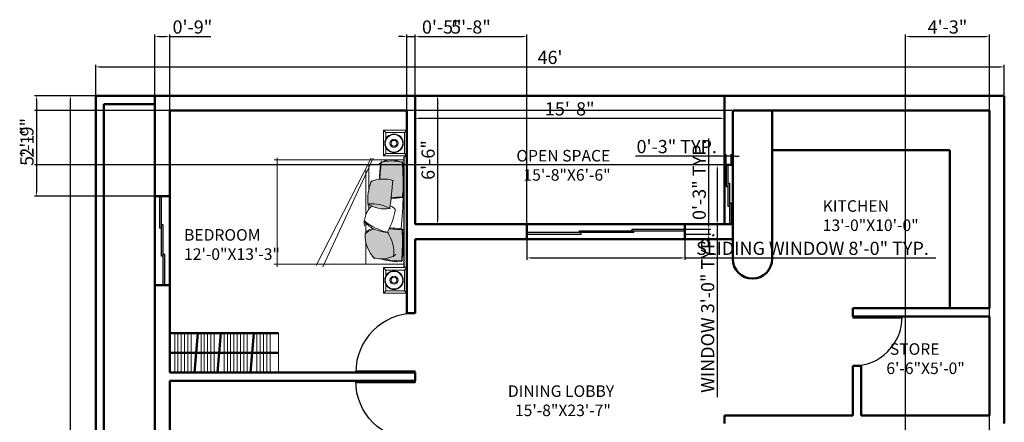
# Model space of a CAD drawing. Units: inches. Extents: x 1913 to 5309, y 1003 to 1733.
# Tile 8 of 23: x 1913 to 2511, y 1489 to 1733. Entities that reach past the tile are written whole.
import ezdxf

# ---------------------------------------------------------------- set-up
doc = ezdxf.new("R2010")
doc.units = ezdxf.units.IN
for name, color, linetype, lineweight in [('0.10', 252, 'Continuous', 9), ('0.15', 34, 'Continuous', 15), ('A-ANNO-DIMS', 2, 'Continuous', 18), ('A-AREA-IDEN', 3, 'Continuous', 18), ('A-DOOR', 4, 'Continuous', 25), ('A-FURN', 8, 'Continuous', 18), ('A-FURN-PATT', 8, 'Continuous', 13), ('A-GLAZ', 5, 'Continuous', 25), ('A-WALL', 7, 'Continuous', 50)]:
    doc.layers.add(name, color=color, linetype=linetype, lineweight=lineweight)
doc.styles.get("Standard").update_dxf_attribs({"font": 'arial.ttf'})
doc.dimstyles.new('ISO-25', dxfattribs={"dimtxt": 8, "dimasz": 2.5, "dimexe": 1.25, "dimexo": 0.625, "dimtad": 1, "dimdec": 1, "dimlunit": 3, "dimtxsty": 'Standard', "dimcen": 2.5, "dimclrd": 256, "dimclrt": 1, "dimadec": 0, "dimazin": 0, "dimtfac": 1, "dimtdec": 1, "dimtmove": 0, "dimatfit": 3, "dimfxl": 1, "dimarcsym": 0})

# ---------------------------------------------------------------- blocks, each defined once
blk = doc.blocks.new("D1 3'")
for p, q in [((0, 36), (0, 0)), ((1, 36), (1, 0)), ((0, 0), (1, 0))]:
    blk.add_line(p, q)
blk.add_arc((0, 0), 36, 0, 90)
blk = doc.blocks.new('camita')
at = {"layer": '0.10'}
for p, q in [((-0.85, -0.045), (0.85, -0.045)), ((-0.805, -0.045), (-0.805, -2.048)), ((0.805, -0.045), (0.805, -2.048)), ((-0.827, -0.521), (0.846, -1.293)), ((-0.827, -0.548), (0.824, -1.399)), ((-0.716, -0.585), (-0.355, -0.585)), ((-0.114, -0.585), (-0.049, -0.585)), ((-0.638, -0.63), (0.043, -0.63)), ((0.175, -0.63), (0.318, -0.63)), ((0.474, -0.63), (0.805, -0.63)), ((-0.835, -2), (0.846, -2))]:
    blk.add_line(p, q, dxfattribs=at)
blk.add_lwpolyline([(-0.85, -0.041), (0.85, -0.041), (0.85, 0), (-0.85, 0)], close=True, dxfattribs=at)
for centre, radius, start, end in [((-0.457, -0.236), 0.344, 147.51, 213.8336), ((-0.2, -0.227), 0.586, 163.9263, 197.1409), ((-0.364, -5.846), 5.791, 83.8073, 94.1211), ((-0.51, -1.723), 1.678, 80.1255, 98.6619), ((2.353, -0.053), 2.58, 180.1063, 184.3854), ((-1.544, -0.245), 1.333, 359.9394, 7.5533), ((1.581, -0.289), 1.335, 170.3802, 178.9914), ((-1.44, -0.061), 1.712, 352.9291, 0.3959), ((0.452, -3.067), 3, 83.9026, 93.6759), ((0.486, -1.629), 1.578, 80.1602, 98.06), ((0.029, -0.138), 0.726, 342.5841, 6.0048), ((0.133, -0.17), 0.631, 339.923, 8.7433), ((-0.054, -0.363), 0.454, 159.3026, 206.5026), ((-1.33, -9.675), 9.499, 82.2708, 84.9399), ((0.458, -0.545), 0.584, 151.0456, 184.1497), ((-0.534, -0.339), 0.487, 327.2644, 9.0473), ((-0.007, -0.258), 0.0828, 100.018, 179.736), ((-0.293, -1.438), 1.29, 61.9749, 77.8435), ((-0.199, -0.274), 0.516, 310.7395, 359.0576), ((-0.567, -0.087), 0.906, 321.6953, 346.4626), ((0.627, -0.752), 0.551, 82.9691, 124.6739), ((0.32, -0.394), 0.404, 341.4524, 33.4512), ((-1.867, -14.986), 14.632, 84.6597, 85.7516), ((-0.46, 1.486), 1.909, 260.953, 268.6517), ((-0.2, 0.064), 0.667, 244.7809, 279.0606), ((0.179, -0.272), 0.383, 224.5284, 275.2229), ((0.438, -0.483), 0.19, 193.6849, 236.7035), ((0.571, -0.432), 0.315, 192.9388, 221.9636), ((0.361, -0.133), 0.51, 267.2589, 315.2997)]:
    blk.add_arc(centre, radius, start, end, dxfattribs=at)
blk = doc.blocks.new('VELADOR')
at = {"layer": '0.15'}
for p, q in [((-0.248, 0), (-0.203, -0.045)), ((0.248, 0), (0.202, -0.045)), ((-0.203, -0.405), (-0.248, -0.45)), ((0.248, -0.45), (0.202, -0.405))]:
    blk.add_line(p, q, dxfattribs=at)
blk.add_lwpolyline([(-0.248, 0), (-0.248, -0.45), (0.248, -0.45), (0.248, 0)], close=True, dxfattribs=at)
blk.add_lwpolyline([(0.092, -0.405), (0.202, -0.405), (0.202, -0.045), (-0.203, -0.045), (-0.203, -0.405), (-0.082, -0.405)], dxfattribs=at)
for radius in [0.18, 0.169, 0.0788, 0.0563]:
    blk.add_circle((0.005, -0.247), radius, dxfattribs=at)
blk = doc.blocks.new('*D20')
at = {"layer": 'A-ANNO-DIMS', "color": 0, "lineweight": -2, "transparency": 16777216}
for p, q in [((1958.75, 1686.96), (1942.76, 1686.96)), ((1944.01, 1101.46), (1944.01, 1684.46)), ((1958.75, 1098.96), (1942.76, 1098.96))]:
    blk.add_line(p, q, dxfattribs=at)
at = {"layer": 'A-ANNO-DIMS', "color": 0, "transparency": 16777216}
for points in [[(1943.6, 1684.46), (1944.43, 1684.46), (1944.01, 1686.96)], [(1943.6, 1101.46), (1944.43, 1101.46), (1944.01, 1098.96)]]:
    blk.add_solid(points, dxfattribs=at)
at = {"layer": 'Defpoints', "color": 0, "transparency": 16777216}
for p in [(1944.01, 1686.96), (1959.37, 1686.96), (1959.37, 1098.96)]:
    blk.add_point(p, dxfattribs=at)
at = {"layer": 'A-ANNO-DIMS', "color": 0, "transparency": 16777216, "insert": (1939.3, 1392.96), "char_height": 8, "attachment_point": 5, "rotation": 90}
blk.add_mtext("49'", dxfattribs=at)
blk = doc.blocks.new('*D22')
at = {"layer": 'A-ANNO-DIMS', "color": 0, "lineweight": -2, "transparency": 16777216}
for p, q in [((1959.37, 1687.59), (1959.37, 1705.75)), ((2511.37, 1687.59), (2511.37, 1705.75)), ((1961.87, 1704.5), (2508.87, 1704.5))]:
    blk.add_line(p, q, dxfattribs=at)
at = {"layer": 'A-ANNO-DIMS', "color": 0, "transparency": 16777216}
for points in [[(1961.87, 1704.92), (1961.87, 1704.08), (1959.37, 1704.5)], [(2508.87, 1704.92), (2508.87, 1704.08), (2511.37, 1704.5)]]:
    blk.add_solid(points, dxfattribs=at)
at = {"layer": 'Defpoints', "color": 0, "transparency": 16777216}
for p in [(2511.37, 1704.5), (1959.37, 1686.96), (2511.37, 1686.96)]:
    blk.add_point(p, dxfattribs=at)
at = {"layer": 'A-ANNO-DIMS', "color": 0, "transparency": 16777216, "insert": (2235.37, 1709.21), "char_height": 8, "attachment_point": 5}
blk.add_mtext("46'", dxfattribs=at)
blk = doc.blocks.new('*D23')
at = {"layer": 'A-ANNO-DIMS', "color": 0, "lineweight": -2, "transparency": 16777216}
for p, q in [((2153.37, 1679.78), (2153.37, 1672.02)), ((2341.37, 1679.78), (2341.37, 1672.02)), ((2155.87, 1673.27), (2338.87, 1673.27))]:
    blk.add_line(p, q, dxfattribs=at)
at = {"layer": 'A-ANNO-DIMS', "color": 0, "transparency": 16777216}
for points in [[(2155.87, 1673.68), (2155.87, 1672.85), (2153.37, 1673.27)], [(2338.87, 1673.68), (2338.87, 1672.85), (2341.37, 1673.27)]]:
    blk.add_solid(points, dxfattribs=at)
at = {"layer": 'Defpoints', "color": 0, "transparency": 16777216}
for p in [(2153.37, 1680.41), (2341.37, 1680.41), (2341.37, 1673.27)]:
    blk.add_point(p, dxfattribs=at)
at = {"layer": 'A-ANNO-DIMS', "color": 0, "transparency": 16777216, "insert": (2247.37, 1677.98), "char_height": 8, "attachment_point": 5}
blk.add_mtext('15\'-8"', dxfattribs=at)
blk = doc.blocks.new('*D24')
at = {"layer": 'A-ANNO-DIMS', "color": 0, "lineweight": -2, "transparency": 16777216}
for p, q in [((2167.19, 1686.96), (2165.81, 1686.96)), ((2167.06, 1684.46), (2167.06, 1611.46)), ((2167.19, 1608.96), (2165.81, 1608.96))]:
    blk.add_line(p, q, dxfattribs=at)
at = {"layer": 'A-ANNO-DIMS', "color": 0, "transparency": 16777216}
for points in [[(2166.65, 1684.46), (2167.48, 1684.46), (2167.06, 1686.96)], [(2166.65, 1611.46), (2167.48, 1611.46), (2167.06, 1608.96)]]:
    blk.add_solid(points, dxfattribs=at)
at = {"layer": 'Defpoints', "color": 0, "transparency": 16777216}
for p in [(2167.81, 1686.96), (2167.06, 1608.96), (2167.81, 1608.96)]:
    blk.add_point(p, dxfattribs=at)
at = {"layer": 'A-ANNO-DIMS', "color": 0, "transparency": 16777216, "insert": (2162.35, 1647.96), "char_height": 8, "attachment_point": 5, "rotation": 90}
blk.add_mtext('6\'-6"', dxfattribs=at)
blk = doc.blocks.new("D2 2'6")
for p, q in [((0, 30), (0, 0)), ((1, 30), (1, 0)), ((0, 0), (1, 0))]:
    blk.add_line(p, q)
blk.add_arc((0, 0), 30, 0, 90)
blk = doc.blocks.new('WIN-54')
for p, q in [((0, 54), (0, 35)), ((1, 54), (1, 17)), ((1, 36), (2, 36)), ((2, 36), (2, 0)), ((0, 35), (1, 35)), ((2, 19), (3, 19)), ((3, 19), (3, 0)), ((1, 17), (2, 17))]:
    blk.add_line(p, q)
blk = doc.blocks.new('WIN-36')
for p, q in [((0, 23), (0, 36)), ((1, 11), (1, 36)), ((2, 25), (1, 25)), ((2, 0), (2, 25)), ((1, 23), (0, 23)), ((3, 13), (2, 13)), ((3, 0), (3, 13)), ((2, 11), (1, 11))]:
    blk.add_line(p, q)
blk = doc.blocks.new('WIN-SLIDER-96')
for p, q in [((65, 1), (0, 1)), ((0, 0), (33, 0)), ((32, 2), (96, 2)), ((32, 1), (32, 2)), ((33, 0), (33, 1)), ((64, 3), (96, 3)), ((64, 2), (64, 3)), ((65, 1), (65, 2))]:
    blk.add_line(p, q)
blk = doc.blocks.new('*D69')
at = {"layer": 'A-ANNO-DIMS', "color": 0, "lineweight": -2, "transparency": 16777216}
for p, q in [((2341.75, 1644.96), (2335.72, 1644.96)), ((2341.75, 1608.96), (2335.72, 1608.96))]:
    blk.add_line(p, q, dxfattribs=at)
at = {"layer": 'A-ANNO-DIMS', "lineweight": -2, "transparency": 16777216}
for p, q in [((2336.97, 1642.46), (2336.97, 1611.46)), ((2336.97, 1608.96), (2336.97, 1503.98))]:
    blk.add_line(p, q, dxfattribs=at)
at = {"layer": 'A-ANNO-DIMS', "transparency": 16777216}
for points in [[(2336.56, 1642.46), (2337.39, 1642.46), (2336.97, 1644.96)], [(2336.56, 1611.46), (2337.39, 1611.46), (2336.97, 1608.96)]]:
    blk.add_solid(points, dxfattribs=at)
at = {"layer": 'Defpoints', "color": 0, "transparency": 16777216}
for p in [(2342.37, 1644.96), (2336.97, 1608.96), (2342.37, 1608.96)]:
    blk.add_point(p, dxfattribs=at)
at = {"layer": 'A-ANNO-DIMS', "color": 1, "transparency": 16777216, "insert": (2332.21, 1555.22), "char_height": 8, "attachment_point": 5, "rotation": 90}
blk.add_mtext('WINDOW 3\'-0" TYP.', dxfattribs=at)
blk = doc.blocks.new('*D70')
at = {"layer": 'A-ANNO-DIMS', "color": 0, "lineweight": -2, "transparency": 16777216}
for p, q in [((2342.37, 1645.59), (2342.37, 1651.61)), ((2345.37, 1645.59), (2345.37, 1651.61))]:
    blk.add_line(p, q, dxfattribs=at)
at = {"layer": 'A-ANNO-DIMS', "lineweight": -2, "transparency": 16777216}
for p, q in [((2339.87, 1650.36), (2287.36, 1650.36)), ((2345.37, 1650.36), (2342.37, 1650.36)), ((2347.87, 1650.36), (2350.37, 1650.36))]:
    blk.add_line(p, q, dxfattribs=at)
at = {"layer": 'A-ANNO-DIMS', "transparency": 16777216}
for points in [[(2339.87, 1650.78), (2339.87, 1649.95), (2342.37, 1650.36)], [(2347.87, 1650.78), (2347.87, 1649.95), (2345.37, 1650.36)]]:
    blk.add_solid(points, dxfattribs=at)
at = {"layer": 'Defpoints', "color": 0, "transparency": 16777216}
for p in [(2342.37, 1650.36), (2342.37, 1644.96), (2345.37, 1644.96)]:
    blk.add_point(p, dxfattribs=at)
at = {"layer": 'A-ANNO-DIMS', "color": 1, "transparency": 16777216, "insert": (2312.37, 1655.08), "char_height": 8, "attachment_point": 5}
blk.add_mtext('0\'-3" TYP.', dxfattribs=at)
blk = doc.blocks.new('*D79')
at = {"layer": 'A-ANNO-DIMS', "color": 0, "lineweight": -2, "transparency": 16777216}
for p, q in [((2221.37, 1602.34), (2221.37, 1587.31)), ((2317.37, 1602.34), (2317.37, 1587.31))]:
    blk.add_line(p, q, dxfattribs=at)
at = {"layer": 'A-ANNO-DIMS', "lineweight": -2, "transparency": 16777216}
for p, q in [((2223.87, 1588.56), (2314.87, 1588.56)), ((2317.37, 1588.56), (2469.81, 1588.56))]:
    blk.add_line(p, q, dxfattribs=at)
at = {"layer": 'A-ANNO-DIMS', "transparency": 16777216}
for points in [[(2223.87, 1588.98), (2223.87, 1588.15), (2221.37, 1588.56)], [(2314.87, 1588.98), (2314.87, 1588.15), (2317.37, 1588.56)]]:
    blk.add_solid(points, dxfattribs=at)
at = {"layer": 'Defpoints', "color": 0, "transparency": 16777216}
for p in [(2221.37, 1602.96), (2317.37, 1602.96), (2317.37, 1588.56)]:
    blk.add_point(p, dxfattribs=at)
at = {"layer": 'A-ANNO-DIMS', "color": 1, "transparency": 16777216, "insert": (2394.84, 1593.33), "char_height": 8, "attachment_point": 5}
blk.add_mtext('SLIDING WINDOW 8\'-0" TYP.', dxfattribs=at)
blk = doc.blocks.new('*D80')
at = {"layer": 'A-ANNO-DIMS', "lineweight": -2, "transparency": 16777216}
for p, q in [((2331.77, 1608.46), (2331.77, 1660.98)), ((2331.77, 1602.96), (2331.77, 1605.96)), ((2331.77, 1600.46), (2331.77, 1597.96))]:
    blk.add_line(p, q, dxfattribs=at)
at = {"layer": 'A-ANNO-DIMS', "color": 0, "lineweight": -2, "transparency": 16777216}
for p, q in [((2318, 1605.96), (2333.02, 1605.96)), ((2318, 1602.96), (2333.02, 1602.96))]:
    blk.add_line(p, q, dxfattribs=at)
at = {"layer": 'A-ANNO-DIMS', "transparency": 16777216}
for points in [[(2331.36, 1608.46), (2332.19, 1608.46), (2331.77, 1605.96)], [(2331.36, 1600.46), (2332.19, 1600.46), (2331.77, 1602.96)]]:
    blk.add_solid(points, dxfattribs=at)
at = {"layer": 'Defpoints', "color": 0, "transparency": 16777216}
for p in [(2317.37, 1605.96), (2331.77, 1605.96), (2317.37, 1602.96)]:
    blk.add_point(p, dxfattribs=at)
at = {"layer": 'A-ANNO-DIMS', "color": 1, "transparency": 16777216, "insert": (2327.06, 1635.97), "char_height": 8, "attachment_point": 5, "rotation": 90}
blk.add_mtext('0\'-3" TYP.', dxfattribs=at)
blk = doc.blocks.new('*D89')
at = {"layer": 'A-ANNO-DIMS', "color": 0, "lineweight": -2, "transparency": 16777216}
for p, q in [((1995.37, 1687.59), (1995.37, 1724.21)), ((2004.37, 1678.59), (2004.37, 1724.21))]:
    blk.add_line(p, q, dxfattribs=at)
at = {"layer": 'A-ANNO-DIMS', "lineweight": -2, "transparency": 16777216}
for p, q in [((1997.87, 1722.96), (2001.87, 1722.96)), ((2004.37, 1722.96), (2029.39, 1722.96))]:
    blk.add_line(p, q, dxfattribs=at)
at = {"layer": 'A-ANNO-DIMS', "transparency": 16777216}
for points in [[(1997.87, 1723.38), (1997.87, 1722.55), (1995.37, 1722.96)], [(2001.87, 1723.38), (2001.87, 1722.55), (2004.37, 1722.96)]]:
    blk.add_solid(points, dxfattribs=at)
at = {"layer": 'Defpoints', "color": 0, "transparency": 16777216}
for p in [(2004.37, 1722.96), (1995.37, 1686.96), (2004.37, 1677.96)]:
    blk.add_point(p, dxfattribs=at)
at = {"layer": 'A-ANNO-DIMS', "color": 1, "transparency": 16777216, "insert": (2018.13, 1727.67), "char_height": 8, "attachment_point": 5}
blk.add_mtext('0\'-9"', dxfattribs=at)
blk = doc.blocks.new('*D90')
at = {"layer": 'A-ANNO-DIMS', "lineweight": -2, "transparency": 16777216}
for p, q in [((2145.87, 1722.96), (2143.37, 1722.96)), ((2148.37, 1722.96), (2153.37, 1722.96)), ((2155.87, 1722.96), (2180.89, 1722.96))]:
    blk.add_line(p, q, dxfattribs=at)
at = {"layer": 'A-ANNO-DIMS', "color": 0, "lineweight": -2, "transparency": 16777216}
for p, q in [((2148.37, 1678.59), (2148.37, 1724.21)), ((2153.37, 1687.59), (2153.37, 1724.21))]:
    blk.add_line(p, q, dxfattribs=at)
at = {"layer": 'A-ANNO-DIMS', "transparency": 16777216}
for points in [[(2145.87, 1723.38), (2145.87, 1722.55), (2148.37, 1722.96)], [(2155.87, 1723.38), (2155.87, 1722.55), (2153.37, 1722.96)]]:
    blk.add_solid(points, dxfattribs=at)
at = {"layer": 'Defpoints', "color": 0, "transparency": 16777216}
for p in [(2153.37, 1722.96), (2153.37, 1686.96), (2148.37, 1677.96)]:
    blk.add_point(p, dxfattribs=at)
at = {"layer": 'A-ANNO-DIMS', "color": 1, "transparency": 16777216, "insert": (2169.63, 1727.67), "char_height": 8, "attachment_point": 5}
blk.add_mtext('0\'-5"', dxfattribs=at)
blk = doc.blocks.new('*D91')
at = {"layer": 'A-ANNO-DIMS', "color": 0, "lineweight": -2, "transparency": 16777216}
for p, q in [((1994.75, 1686.96), (1922.12, 1686.96)), ((1994.75, 1625.96), (1922.12, 1625.96))]:
    blk.add_line(p, q, dxfattribs=at)
at = {"layer": 'A-ANNO-DIMS', "lineweight": -2, "transparency": 16777216}
blk.add_line((1923.37, 1684.46), (1923.37, 1628.46), dxfattribs=at)
at = {"layer": 'A-ANNO-DIMS', "transparency": 16777216}
for points in [[(1922.96, 1684.46), (1923.79, 1684.46), (1923.37, 1686.96)], [(1922.96, 1628.46), (1923.79, 1628.46), (1923.37, 1625.96)]]:
    blk.add_solid(points, dxfattribs=at)
at = {"layer": 'Defpoints', "color": 0, "transparency": 16777216}
for p in [(1995.37, 1686.96), (1923.37, 1625.96), (1995.37, 1625.96)]:
    blk.add_point(p, dxfattribs=at)
at = {"layer": 'A-ANNO-DIMS', "color": 1, "transparency": 16777216, "insert": (1918.66, 1656.46), "char_height": 8, "attachment_point": 5, "rotation": 90}
blk.add_mtext('5\'-1"', dxfattribs=at)
blk = doc.blocks.new('*D93')
at = {"layer": 'A-ANNO-DIMS', "color": 0, "lineweight": -2, "transparency": 16777216}
for p, q in [((2345.75, 1677.96), (1922.12, 1677.96)), ((2345.75, 1644.96), (1922.12, 1644.96))]:
    blk.add_line(p, q, dxfattribs=at)
at = {"layer": 'A-ANNO-DIMS', "lineweight": -2, "transparency": 16777216}
blk.add_line((1923.37, 1675.46), (1923.37, 1647.46), dxfattribs=at)
at = {"layer": 'A-ANNO-DIMS', "transparency": 16777216}
for points in [[(1922.96, 1675.46), (1923.79, 1675.46), (1923.37, 1677.96)], [(1922.96, 1647.46), (1923.79, 1647.46), (1923.37, 1644.96)]]:
    blk.add_solid(points, dxfattribs=at)
at = {"layer": 'Defpoints', "color": 0, "transparency": 16777216}
for p in [(2346.37, 1677.96), (1923.37, 1644.96), (2346.37, 1644.96)]:
    blk.add_point(p, dxfattribs=at)
at = {"layer": 'A-ANNO-DIMS', "color": 1, "transparency": 16777216, "insert": (1918.66, 1661.46), "char_height": 8, "attachment_point": 5, "rotation": 90}
blk.add_mtext('2\'-9"', dxfattribs=at)
blk = doc.blocks.new('*D94')
at = {"layer": 'A-ANNO-DIMS', "color": 0, "lineweight": -2, "transparency": 16777216}
for p, q in [((2153.37, 1609.59), (2153.37, 1724.21)), ((2221.37, 1609.59), (2221.37, 1724.21))]:
    blk.add_line(p, q, dxfattribs=at)
at = {"layer": 'A-ANNO-DIMS', "lineweight": -2, "transparency": 16777216}
blk.add_line((2155.87, 1722.96), (2218.87, 1722.96), dxfattribs=at)
at = {"layer": 'A-ANNO-DIMS', "transparency": 16777216}
for points in [[(2155.87, 1723.38), (2155.87, 1722.55), (2153.37, 1722.96)], [(2218.87, 1723.38), (2218.87, 1722.55), (2221.37, 1722.96)]]:
    blk.add_solid(points, dxfattribs=at)
at = {"layer": 'Defpoints', "color": 0, "transparency": 16777216}
for p in [(2221.37, 1722.96), (2153.37, 1608.96), (2221.37, 1608.96)]:
    blk.add_point(p, dxfattribs=at)
at = {"layer": 'A-ANNO-DIMS', "color": 1, "transparency": 16777216, "insert": (2187.37, 1727.67), "char_height": 8, "attachment_point": 5}
blk.add_mtext('5\'-8"', dxfattribs=at)
blk = doc.blocks.new('*D99')
at = {"layer": 'A-ANNO-DIMS', "color": 0, "lineweight": -2, "transparency": 16777216}
for p, q in [((2451.37, 1180.59), (2451.37, 1724.21)), ((2502.37, 1180.59), (2502.37, 1724.21))]:
    blk.add_line(p, q, dxfattribs=at)
at = {"layer": 'A-ANNO-DIMS', "lineweight": -2, "transparency": 16777216}
blk.add_line((2453.87, 1722.96), (2499.87, 1722.96), dxfattribs=at)
at = {"layer": 'A-ANNO-DIMS', "transparency": 16777216}
for points in [[(2453.87, 1723.38), (2453.87, 1722.55), (2451.37, 1722.96)], [(2499.87, 1723.38), (2499.87, 1722.55), (2502.37, 1722.96)]]:
    blk.add_solid(points, dxfattribs=at)
at = {"layer": 'Defpoints', "color": 0, "transparency": 16777216}
for p in [(2502.37, 1722.96), (2451.37, 1179.96), (2502.37, 1179.96)]:
    blk.add_point(p, dxfattribs=at)
at = {"layer": 'A-ANNO-DIMS', "color": 1, "transparency": 16777216, "insert": (2476.87, 1727.68), "char_height": 8, "attachment_point": 5}
blk.add_mtext('4\'-3"', dxfattribs=at)

msp = doc.modelspace()

# ---------------------------------------------------------------- hatches: boundary and pattern name
at = {"layer": 'A-FURN-PATT'}
h = msp.add_hatch(color=256, dxfattribs=at)
h.dxf.hatch_style = 1
h.paths.add_polyline_path([(2131.94, 1636.36, -0.113891), (2139.94, 1635.49, -0.006967), (2138.87, 1625.13, -0.016701), (2145.65, 1625.4, 0.015442), (2146.21, 1629.44, 0.01851), (2145.69, 1646.31, 0.020657), (2144.69, 1646.81, 0.131047), (2132.8, 1646.43, -0.004387)])
h.paths.add_polyline_path([(2137.68, 1606.26, -0.011742), (2136.61, 1604.13, -0.175864), (2140.37, 1589.82, -0.098488), (2134.43, 1588.01, 0.094792), (2145.1, 1586.79, 0.040212), (2145.49, 1605.75, -0.029051)])
h = msp.add_hatch(color=256, dxfattribs=at)
h.dxf.hatch_style = 1
h.paths.add_polyline_path([(2124.8, 1621.24, 0.181694), (2138.03, 1618.54, 0.011408), (2139.94, 1635.49, 0.189536), (2126.86, 1634.97, 0.134508)])
h.paths.add_polyline_path([(2136.7, 1603.99, -0.104045), (2128.6, 1606.06, 0.127326), (2123.09, 1603.2, 0.202559), (2128.48, 1588.54, 0.194952), (2140.37, 1589.82, 0.173835)])

# ---------------------------------------------------------------- linework, layer by layer
at = {"layer": 'A-FURN'}
for p, q in [((2007.37, 1542.96), (2007.37, 1518.96)), ((2009.37, 1542.96), (2009.37, 1518.96)), ((2011.37, 1542.96), (2011.37, 1518.96)), ((2013.37, 1542.96), (2013.37, 1518.96)), ((2015.37, 1542.96), (2015.37, 1518.96)), ((2017.37, 1542.96), (2017.37, 1518.96)), ((2023.37, 1542.96), (2023.37, 1518.96)), ((2025.37, 1542.96), (2025.37, 1518.96)), ((2027.37, 1542.96), (2027.37, 1518.96)), ((2029.37, 1542.96), (2029.37, 1518.96)), ((2031.37, 1542.96), (2031.37, 1518.96)), ((2037.37, 1542.96), (2037.37, 1518.96)), ((2039.37, 1542.96), (2039.37, 1518.96)), ((2041.37, 1542.96), (2041.37, 1518.96)), ((2043.37, 1542.96), (2043.37, 1518.96)), ((2045.37, 1542.96), (2045.37, 1518.96)), ((2047.37, 1542.96), (2047.37, 1518.96)), ((2049.37, 1542.96), (2049.37, 1518.96)), ((2051.37, 1542.96), (2051.37, 1518.96)), ((2057.37, 1542.96), (2057.37, 1518.96)), ((2059.37, 1542.96), (2059.37, 1518.96)), ((2061.37, 1542.96), (2061.37, 1518.96)), ((2063.37, 1542.96), (2063.37, 1518.96)), ((2065.37, 1542.96), (2065.37, 1518.96)), ((2070.37, 1542.96), (2070.37, 1518.96))]:
    msp.add_line(p, q, dxfattribs=at)
at = {"layer": 'A-WALL'}
for p, q in [((1959.37, 1686.96), (2511.37, 1686.96)), ((1959.37, 1098.96), (1959.37, 1686.96)), ((1995.37, 1686.96), (1995.37, 1420.96)), ((2153.37, 1686.96), (2153.37, 1608.96)), ((2341.37, 1686.96), (2341.37, 1608.96)), ((2511.37, 1686.96), (2511.37, 1487.96)), ((1964.37, 1103.96), (1964.37, 1681.96)), ((1964.37, 1681.96), (1995.37, 1681.96)), ((2004.37, 1677.96), (2148.37, 1677.96)), ((2004.37, 1677.96), (2004.37, 1518.96)), ((2148.37, 1677.96), (2148.37, 1554.96)), ((2346.37, 1677.96), (2502.37, 1677.96)), ((2346.37, 1677.96), (2346.37, 1587.96)), ((2370.37, 1677.96), (2370.37, 1587.96)), ((2502.37, 1677.96), (2502.37, 1557.96)), ((2370.37, 1653.96), (2478.37, 1653.96)), ((2478.37, 1653.96), (2478.37, 1557.96)), ((2346.37, 1644.96), (2341.37, 1644.96)), ((1995.37, 1625.96), (2004.37, 1625.96)), ((2153.37, 1608.96), (2341.37, 1608.96)), ((2221.37, 1599.96), (2221.37, 1608.96)), ((2317.37, 1599.96), (2317.37, 1608.96)), ((2346.37, 1608.96), (2341.37, 1608.96)), ((2153.37, 1599.96), (2346.37, 1599.96)), ((2153.37, 1599.96), (2153.37, 1554.96)), ((1995.37, 1571.96), (2004.37, 1571.96)), ((2419.37, 1557.96), (2502.37, 1557.96)), ((2419.37, 1557.96), (2419.37, 1552.96)), ((2148.37, 1554.96), (2153.37, 1554.96)), ((2419.37, 1552.96), (2502.37, 1552.96)), ((2502.37, 1552.96), (2502.37, 1492.96)), ((2004.37, 1542.96), (2070.37, 1542.96)), ((2021.37, 1542.96), (2019.37, 1518.96)), ((2035.37, 1542.96), (2033.37, 1518.96)), ((2055.37, 1542.96), (2053.37, 1518.96)), ((2070.37, 1530.96), (2004.37, 1530.96)), ((2419.37, 1522.96), (2424.37, 1522.96)), ((2419.37, 1522.96), (2419.37, 1492.96)), ((2424.37, 1522.96), (2424.37, 1492.96)), ((2004.37, 1518.96), (2153.37, 1518.96)), ((2004.37, 1513.96), (2004.37, 1429.96)), ((2004.37, 1513.96), (2153.37, 1513.96)), ((2153.37, 1518.96), (2153.37, 1513.96)), ((2341.37, 1492.96), (2341.37, 1487.96)), ((2341.37, 1492.96), (2419.37, 1492.96)), ((2424.37, 1492.96), (2502.37, 1492.96))]:
    msp.add_line(p, q, dxfattribs=at)
msp.add_arc((2358.37, 1587.96), 12, 180, 360, dxfattribs=at)

# ---------------------------------------------------------------- block references
at = {"layer": 'A-DOOR'}
for name, p, rotation in [("D1 3'", (2153.37, 1518.96), 90), ("D2 2'6", (2419.37, 1552.96), 270)]:
    msp.add_blockref(name, p, dxfattribs=dict(at, rotation=rotation))
at = {"layer": 'A-DOOR', "xscale": -1, "rotation": 90}
msp.add_blockref("D1 3'", (2153.37, 1513.96), dxfattribs=at)
at = {"layer": 'A-FURN'}
for name, p, xscale, yscale, zscale, rotation in [('VELADOR', (2148.37, 1658.3), 31.41542173157097, 31.41542173157097, 31.41542173157097, 270), ('camita', (2148.37, 1616.46), 39.375, 39.375, 39.375, 270), ('VELADOR', (2148.37, 1574.85), -31.41542173157097, 31.41542173157097, 31.41542173157097, 269.9999999999999)]:
    msp.add_blockref(name, p, dxfattribs=dict(at, xscale=xscale, yscale=yscale, zscale=zscale, rotation=rotation))
at = {"layer": 'A-GLAZ'}
for name, p, rotation in [('WIN-36', (2345.37, 1644.96), 180), ('WIN-54', (2001.35, 1625.59), 180.0440757868837)]:
    msp.add_blockref(name, p, dxfattribs=dict(at, rotation=rotation))
msp.add_blockref('WIN-SLIDER-96', (2221.37, 1602.96), dxfattribs=at)

# ---------------------------------------------------------------- texts
at = {"layer": 'A-AREA-IDEN', "char_height": 7, "attachment_point": 1}
for s, width, insert in [('OPEN SPACE\\P  15\'-8"X6\'-6"', 115.9003, (2214.96, 1654.08)), ('KITCHEN\\P13\'-0"X10\'-0"', 86.9528, (2401.07, 1623.55)), ('BEDROOM\\P12\'-0"X13\'-3"', 86.9528, (2013.05, 1606.02)), (' STORE\\P6\'-6"X5\'-0"', 86.9528, (2439.69, 1536.74)), ('DINING LOBBY\\P  15\'-8"X23\'-7"', 86.9528, (2209.8, 1511.2))]:
    msp.add_mtext_dynamic_manual_height_columns(s, width=width, gutter_width=12.5, heights=[0], dxfattribs=dict(at, insert=insert))

# ---------------------------------------------------------------- dimensions: what is measured, and where the dimension line sits
at = {"layer": 'A-ANNO-DIMS'}
for base, p1, p2, override, picture, middle in [((2004.37, 1722.96), (1995.37, 1686.96), (2004.37, 1677.96), {"dimdec": 1, "dimlfac": 1, "dimrnd": 0, "dimzin": 1, "dimdsep": 46, "dimlunit": 4, "dimfrac": 2}, '*D89', (2018.13, 1727.67)), ((2153.37, 1722.96), (2148.37, 1677.96), (2153.37, 1686.96), {"dimdec": 1, "dimlfac": 1, "dimrnd": 0, "dimzin": 1, "dimdsep": 46, "dimlunit": 4, "dimfrac": 2}, '*D90', (2169.63, 1727.67)), ((2221.37, 1722.96), (2153.37, 1608.96), (2221.37, 1608.96), {"dimdec": 1, "dimlfac": 1, "dimrnd": 0, "dimzin": 1, "dimdsep": 46, "dimlunit": 4, "dimfrac": 2}, '*D94', (2187.37, 1727.67)), ((2502.37, 1722.96), (2451.37, 1179.96), (2502.37, 1179.96), {"dimdec": 1, "dimlfac": 1, "dimrnd": 0, "dimzin": 1, "dimdsep": 46, "dimlunit": 4, "dimfrac": 2}, '*D99', (2476.87, 1727.68)), ((2511.37, 1704.5), (1959.37, 1686.96), (2511.37, 1686.96), {"dimclrd": 0, "dimclre": 0, "dimclrt": 0}, '*D22', (2235.37, 1709.21)), ((2341.37, 1673.27), (2153.37, 1680.41), (2341.37, 1680.41), {"dimclrd": 0, "dimclre": 0, "dimclrt": 0}, '*D23', (2247.37, 1677.98))]:
    dim = msp.add_linear_dim(base=base, p1=p1, p2=p2, dimstyle='ISO-25', override=override, dxfattribs=at)
    dim.commit()
    dim.dimension.update_dxf_attribs({"geometry": picture, "text_midpoint": middle})
for base, p1, p2, override, picture, middle in [((1923.37, 1625.96), (1995.37, 1686.96), (1995.37, 1625.96), {"dimdec": 1, "dimlfac": 1, "dimrnd": 0, "dimzin": 1, "dimdsep": 46, "dimlunit": 4, "dimfrac": 2}, '*D91', (1918.66, 1656.46)), ((1944.01, 1686.96), (1959.37, 1098.96), (1959.37, 1686.96), {"dimclrd": 0, "dimclre": 0, "dimclrt": 0}, '*D20', (1939.3, 1392.96)), ((2167.06, 1608.96), (2167.81, 1686.96), (2167.81, 1608.96), {"dimclrd": 0, "dimclre": 0, "dimclrt": 0}, '*D24', (2162.35, 1647.96)), ((1923.37, 1644.96), (2346.37, 1677.96), (2346.37, 1644.96), {"dimdec": 1, "dimlfac": 1, "dimrnd": 0, "dimzin": 1, "dimdsep": 46, "dimlunit": 4, "dimfrac": 2}, '*D93', (1918.66, 1661.46))]:
    dim = msp.add_linear_dim(base=base, p1=p1, p2=p2, angle=90, dimstyle='ISO-25', override=override, dxfattribs=at)
    dim.commit()
    dim.dimension.update_dxf_attribs({"geometry": picture, "text_midpoint": middle})
for base, p1, p2, angle, text, picture, middle in [((2342.37, 1650.36), (2345.37, 1644.96), (2342.37, 1644.96), 180, '<> TYP.', '*D70', (2312.37, 1655.08)), ((2331.77, 1605.96), (2317.37, 1602.96), (2317.37, 1605.96), 90, '<> TYP.', '*D80', (2327.06, 1635.97)), ((2336.97, 1608.96), (2342.37, 1644.96), (2342.37, 1608.96), 270, 'WINDOW <> TYP.', '*D69', (2332.21, 1555.22))]:
    dim = msp.add_linear_dim(base=base, p1=p1, p2=p2, angle=angle, text=text, dimstyle='ISO-25', override={"dimdec": 1, "dimrnd": 0, "dimzin": 1, "dimlunit": 4, "dimfrac": 2}, dxfattribs=at)
    dim.commit()
    dim.dimension.update_dxf_attribs({"geometry": picture, "text_midpoint": middle})
dim = msp.add_linear_dim(base=(2317.37, 1588.56), p1=(2221.37, 1602.96), p2=(2317.37, 1602.96), text='SLIDING WINDOW <> TYP.', dimstyle='ISO-25', override={"dimdec": 1, "dimrnd": 0, "dimzin": 1, "dimlunit": 4, "dimfrac": 2}, dxfattribs=at)
dim.commit()
dim.dimension.update_dxf_attribs({"geometry": '*D79', "text_midpoint": (2394.84, 1593.33)})

doc.saveas('drawing.dxf')
